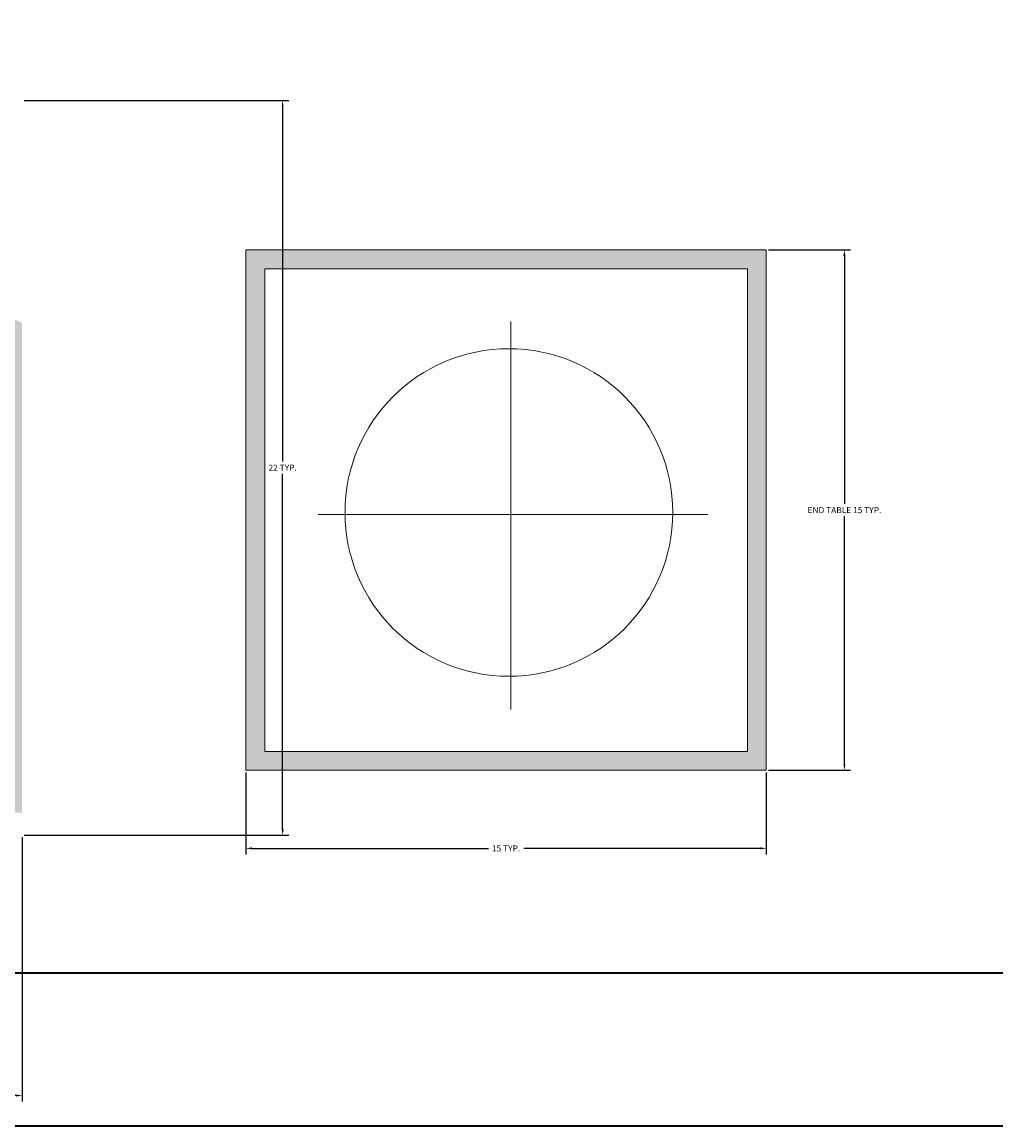
# Model space of a CAD drawing. Units: millimetres. Extents: x 27017497 to 27018854, y 7058029 to 7059154.
# Tile 53 of 91: x 27017980 to 27018009, y 7058294 to 7058327. Entities that reach past the tile are written whole.
import ezdxf

# ---------------------------------------------------------------- set-up
doc = ezdxf.new("R2010")
doc.units = ezdxf.units.MM
for name, color, linetype, lineweight in [('A-ANNO-DIMS', 2, 'Continuous', 18), ('A-FURN', 8, 'Continuous', 18), ('A-WALL', 7, 'Continuous', 35)]:
    doc.layers.add(name, color=color, linetype=linetype, lineweight=lineweight)
doc.layers.add('A-FURN-PATT', color=177, linetype='Continuous', lineweight=13, true_color=0x293189)
doc.styles.get("Standard").update_dxf_attribs({"font": 'arial.ttf'})
doc.dimstyles.get("Standard").update_dxf_attribs({"dimtxt": 0.18, "dimasz": 0.18, "dimexe": 0.18, "dimexo": 0.0625, "dimgap": 0.09, "dimtad": 0, "dimtih": 1, "dimtoh": 1, "dimdec": 4, "dimzin": 0, "dimdsep": 46, "dimtxsty": 'Standard', "dimcen": 0.09, "dimadec": 0, "dimazin": 0, "dimtfac": 1, "dimtdec": 4, "dimtofl": 0, "dimtmove": 0, "dimatfit": 3, "dimfxl": 1, "dimtolj": 1, "dimtzin": 0, "dimarcsym": 0})

# ---------------------------------------------------------------- blocks, each defined once
blk = doc.blocks.new('TABLE-END')
for p, q in [((15.283, 15.283), (0, 15.283)), ((0, 15.283), (0, 0)), ((15.283, 0), (15.283, 15.283)), ((14.727, 14.727), (0.555, 14.727)), ((0.555, 14.727), (0.555, 0.555)), ((14.727, 0.555), (14.727, 14.727)), ((7.785, 1.782), (7.785, 13.175)), ((2.122, 7.509), (13.57, 7.509)), ((0.555, 0.555), (14.727, 0.555)), ((0, 0), (15.283, 0))]:
    blk.add_line(p, q)
blk.add_circle((7.724, 7.57), 4.811)
blk = doc.blocks.new('*D29')
at = {"layer": 'A-ANNO-DIMS', "color": 0, "lineweight": -2, "transparency": 16777216}
for p, q in [((27018002.294, 7058320.14), (27018004.704, 7058320.14)), ((27018004.524, 7058319.96), (27018004.524, 7058312.68)), ((27018004.524, 7058305.037), (27018004.524, 7058312.316)), ((27018002.294, 7058304.857), (27018004.704, 7058304.857))]:
    blk.add_line(p, q, dxfattribs=at)
at = {"layer": 'A-ANNO-DIMS', "color": 0, "transparency": 16777216}
for points in [[(27018004.494, 7058319.96), (27018004.554, 7058319.96), (27018004.524, 7058320.14)], [(27018004.494, 7058305.037), (27018004.554, 7058305.037), (27018004.524, 7058304.857)]]:
    blk.add_solid(points, dxfattribs=at)
at = {"layer": 'Defpoints', "color": 0, "transparency": 16777216}
for p in [(27018002.231, 7058320.14), (27018004.524, 7058320.14), (27018002.231, 7058304.857)]:
    blk.add_point(p, dxfattribs=at)
at = {"layer": 'A-ANNO-DIMS', "color": 0, "transparency": 16777216, "insert": (27018004.524, 7058312.498), "char_height": 0.18, "attachment_point": 5}
blk.add_mtext('\\A1;END TABLE 15 TYP.', dxfattribs=at)
blk = doc.blocks.new('*D30')
at = {"layer": 'A-ANNO-DIMS', "color": 0, "lineweight": -2, "transparency": 16777216}
for p, q in [((27017986.948, 7058304.794), (27017986.948, 7058302.384)), ((27018002.231, 7058304.794), (27018002.231, 7058302.384)), ((27017987.128, 7058302.564), (27017994.07, 7058302.564)), ((27018002.051, 7058302.564), (27017995.109, 7058302.564))]:
    blk.add_line(p, q, dxfattribs=at)
at = {"layer": 'A-ANNO-DIMS', "color": 0, "transparency": 16777216}
for points in [[(27017987.128, 7058302.594), (27017987.128, 7058302.534), (27017986.948, 7058302.564)], [(27018002.051, 7058302.594), (27018002.051, 7058302.534), (27018002.231, 7058302.564)]]:
    blk.add_solid(points, dxfattribs=at)
at = {"layer": 'Defpoints', "color": 0, "transparency": 16777216}
for p in [(27017986.948, 7058304.857), (27018002.231, 7058304.857), (27018002.231, 7058302.564)]:
    blk.add_point(p, dxfattribs=at)
at = {"layer": 'A-ANNO-DIMS', "color": 0, "transparency": 16777216, "insert": (27017994.59, 7058302.564), "char_height": 0.18, "attachment_point": 5}
blk.add_mtext('\\A1;15 TYP.', dxfattribs=at)
blk = doc.blocks.new('*D37')
at = {"layer": 'A-ANNO-DIMS', "color": 0, "lineweight": -2, "transparency": 16777216}
for p, q in [((27017929.382, 7058302.892), (27017929.382, 7058295.125)), ((27017980.38, 7058302.892), (27017980.38, 7058295.125)), ((27017929.562, 7058295.305), (27017953.976, 7058295.305)), ((27017980.2, 7058295.305), (27017955.786, 7058295.305))]:
    blk.add_line(p, q, dxfattribs=at)
at = {"layer": 'A-ANNO-DIMS', "color": 0, "transparency": 16777216}
for points in [[(27017929.562, 7058295.335), (27017929.562, 7058295.275), (27017929.382, 7058295.305)], [(27017980.2, 7058295.335), (27017980.2, 7058295.275), (27017980.38, 7058295.305)]]:
    blk.add_solid(points, dxfattribs=at)
at = {"layer": 'Defpoints', "color": 0, "transparency": 16777216}
for p in [(27017929.382, 7058302.955), (27017980.38, 7058302.955), (27017980.38, 7058295.305)]:
    blk.add_point(p, dxfattribs=at)
at = {"layer": 'A-ANNO-DIMS', "color": 0, "transparency": 16777216, "insert": (27017954.881, 7058295.305), "char_height": 0.18, "attachment_point": 5}
blk.add_mtext('\\A1;SOFA 51 TYP.', dxfattribs=at)
blk = doc.blocks.new('*D38')
at = {"layer": 'A-ANNO-DIMS', "color": 0, "lineweight": -2, "transparency": 16777216}
for p, q in [((27017980.443, 7058324.531), (27017988.21, 7058324.531)), ((27017988.03, 7058324.351), (27017988.03, 7058313.923)), ((27017988.03, 7058303.135), (27017988.03, 7058313.562)), ((27017980.443, 7058302.955), (27017988.21, 7058302.955))]:
    blk.add_line(p, q, dxfattribs=at)
at = {"layer": 'A-ANNO-DIMS', "color": 0, "transparency": 16777216}
for points in [[(27017988, 7058324.351), (27017988.06, 7058324.351), (27017988.03, 7058324.531)], [(27017988, 7058303.135), (27017988.06, 7058303.135), (27017988.03, 7058302.955)]]:
    blk.add_solid(points, dxfattribs=at)
at = {"layer": 'Defpoints', "color": 0, "transparency": 16777216}
for p in [(27017980.38, 7058324.531), (27017988.03, 7058324.531), (27017980.38, 7058302.955)]:
    blk.add_point(p, dxfattribs=at)
at = {"layer": 'A-ANNO-DIMS', "color": 0, "transparency": 16777216, "insert": (27017988.03, 7058313.743), "char_height": 0.18, "attachment_point": 5}
blk.add_mtext('\\A1;22 TYP.', dxfattribs=at)
blk = doc.blocks.new('*D48')
at = {"layer": 'A-ANNO-DIMS', "color": 0, "lineweight": -2, "transparency": 16777216}
for p, q in [((27018463.498, 7058622.912), (27017497.536, 7058622.912)), ((27017497.716, 7058622.732), (27017497.716, 7058357.753)), ((27017497.716, 7058092.41), (27017497.716, 7058357.389)), ((27018555.129, 7058092.23), (27017497.536, 7058092.23))]:
    blk.add_line(p, q, dxfattribs=at)
at = {"layer": 'A-ANNO-DIMS', "color": 0, "transparency": 16777216}
for points in [[(27017497.686, 7058622.732), (27017497.746, 7058622.732), (27017497.716, 7058622.912)], [(27017497.686, 7058092.41), (27017497.746, 7058092.41), (27017497.716, 7058092.23)]]:
    blk.add_solid(points, dxfattribs=at)
at = {"layer": 'Defpoints', "color": 0, "transparency": 16777216}
for p in [(27018463.561, 7058622.912), (27017497.716, 7058092.23), (27018555.192, 7058092.23)]:
    blk.add_point(p, dxfattribs=at)
at = {"layer": 'A-ANNO-DIMS', "color": 0, "transparency": 16777216, "insert": (27017497.716, 7058357.571), "char_height": 0.18, "attachment_point": 5}
blk.add_mtext('\\A1;530.7', dxfattribs=at)

msp = doc.modelspace()

# ---------------------------------------------------------------- hatches: boundary and pattern name
at = {"layer": 'A-FURN-PATT'}
h = msp.add_hatch(color=256, dxfattribs=at)
h.dxf.hatch_style = 1
h.paths.add_polyline_path([(27017972.67, 7058349.702), (27017940.993, 7058349.702), (27017940.993, 7058334.697), (27017972.67, 7058334.697)])
h.paths.add_polyline_path([(27017962.073, 7058324.531), (27017947.689, 7058324.531), (27017947.689, 7058312.108), (27017962.073, 7058312.108)])
h.paths.add_polyline_path([(27017977.111, 7058320.608), (27017977.111, 7058324.531), (27017962.073, 7058324.531), (27017962.073, 7058312.108), (27017977.111, 7058312.108), (27017977.111, 7058317.992)])
h.paths.add_polyline_path([(27017947.689, 7058324.531), (27017932.651, 7058324.531), (27017932.651, 7058320.608), (27017932.651, 7058317.992), (27017932.651, 7058312.108), (27017947.689, 7058312.108)])
h.paths.add_polyline_path([(27017932.651, 7058317.992), (27017931.997, 7058318.646), (27017930.69, 7058318.646), (27017929.382, 7058317.992), (27017929.382, 7058303.608), (27017932.651, 7058303.608), (27017932.651, 7058302.955), (27017977.111, 7058302.955), (27017977.111, 7058303.608), (27017980.38, 7058303.608), (27017980.38, 7058317.992), (27017979.072, 7058318.646), (27017977.765, 7058318.646), (27017977.111, 7058317.992), (27017977.111, 7058304.916), (27017932.651, 7058304.916)])
h.paths.add_polyline_path([(27017947.689, 7058312.108), (27017932.651, 7058312.108), (27017932.651, 7058310.8), (27017947.689, 7058310.8)], flags=17)
h.paths.add_polyline_path([(27017962.073, 7058312.108), (27017947.689, 7058312.108), (27017947.689, 7058310.8), (27017962.073, 7058310.8)], flags=17)
h.paths.add_polyline_path([(27017977.111, 7058312.108), (27017962.073, 7058312.108), (27017962.073, 7058310.8), (27017977.111, 7058310.8)], flags=17)
h.paths.add_polyline_path([(27017977.111, 7058310.8), (27017962.073, 7058310.8), (27017962.073, 7058309.493), (27017977.111, 7058309.493)], flags=17)
h.paths.add_polyline_path([(27017962.073, 7058310.8), (27017947.689, 7058310.8), (27017947.689, 7058309.493), (27017962.073, 7058309.493)], flags=17)
h.paths.add_polyline_path([(27017947.689, 7058310.8), (27017932.651, 7058310.8), (27017932.651, 7058309.493), (27017947.689, 7058309.493)], flags=17)
h.paths.add_polyline_path([(27017947.689, 7058309.493), (27017932.651, 7058309.493), (27017932.651, 7058304.916), (27017947.689, 7058304.916)], flags=17)
h.paths.add_polyline_path([(27017962.073, 7058309.493), (27017947.689, 7058309.493), (27017947.689, 7058304.916), (27017962.073, 7058304.916)], flags=17)
h.paths.add_polyline_path([(27017977.111, 7058309.493), (27017962.073, 7058309.493), (27017962.073, 7058304.916), (27017977.111, 7058304.916)], flags=17)
h.paths.add_polyline_path([(27017979.072, 7058320.608), (27017977.111, 7058320.608), (27017977.111, 7058317.992), (27017977.765, 7058318.646), (27017979.072, 7058318.646)])
h.paths.add_polyline_path([(27017932.651, 7058320.608), (27017930.69, 7058320.608), (27017930.69, 7058318.646), (27017931.997, 7058318.646), (27017932.651, 7058317.992)])
h.paths.add_polyline_path([(27018002.231, 7058320.14), (27017986.948, 7058320.14), (27017986.948, 7058304.857), (27018002.231, 7058304.857)])
h.paths.add_polyline_path([(27018001.676, 7058319.584), (27018001.676, 7058305.412), (27017987.504, 7058305.412), (27017987.504, 7058319.584)], flags=16)
h.paths.add_polyline_path([(27017999.483, 7058312.427, -1), (27017989.862, 7058312.427, -1)], flags=0)

# ---------------------------------------------------------------- linework, layer by layer
at = {"layer": 'A-WALL'}
for p, q in [((27017888.166, 7058298.912), (27018032.166, 7058298.912)), ((27017888.166, 7058294.412), (27018032.166, 7058294.412))]:
    msp.add_line(p, q, dxfattribs=at)

# ---------------------------------------------------------------- block references
at = {"layer": 'A-FURN'}
msp.add_blockref('TABLE-END', (27017986.948, 7058304.857), dxfattribs=at)

# ---------------------------------------------------------------- dimensions: what is measured, and where the dimension line sits
at = {"layer": 'A-ANNO-DIMS'}
dim = msp.add_linear_dim(base=(27017497.716, 7058092.23), p1=(27018463.561, 7058622.912), p2=(27018555.192, 7058092.23), angle=90, dimstyle='Standard', override={"dimdec": 1, "dimlfac": 1, "dimrnd": 0, "dimzin": 0, "dimdsep": 46, "dimlunit": 2}, dxfattribs=at)
dim.commit()
dim.dimension.update_dxf_attribs({"geometry": '*D48', "text_midpoint": (27017497.716, 7058357.571)})
for base, p1, p2, text, picture, middle in [((27017988.03, 7058324.531), (27017980.38, 7058302.955), (27017980.38, 7058324.531), '<> TYP.', '*D38', (27017988.03, 7058313.743)), ((27018004.524, 7058320.14), (27018002.231, 7058304.857), (27018002.231, 7058320.14), 'END TABLE <> TYP.', '*D29', (27018004.524, 7058312.498))]:
    dim = msp.add_linear_dim(base=base, p1=p1, p2=p2, angle=90, text=text, dimstyle='Standard', override={"dimdec": 0, "dimlfac": 1, "dimrnd": 0, "dimzin": 0, "dimdsep": 46, "dimlunit": 2}, dxfattribs=at)
    dim.commit()
    dim.dimension.update_dxf_attribs({"geometry": picture, "text_midpoint": middle})
for base, p1, p2, text, picture, middle in [((27018002.231, 7058302.564), (27017986.948, 7058304.857), (27018002.231, 7058304.857), '<> TYP.', '*D30', (27017994.59, 7058302.564)), ((27017980.38, 7058295.305), (27017929.382, 7058302.955), (27017980.38, 7058302.955), 'SOFA <> TYP.', '*D37', (27017954.881, 7058295.305))]:
    dim = msp.add_linear_dim(base=base, p1=p1, p2=p2, text=text, dimstyle='Standard', override={"dimdec": 0, "dimlfac": 1, "dimrnd": 0, "dimzin": 0, "dimdsep": 46, "dimlunit": 2}, dxfattribs=at)
    dim.commit()
    dim.dimension.update_dxf_attribs({"geometry": picture, "text_midpoint": middle})

doc.saveas('drawing.dxf')
